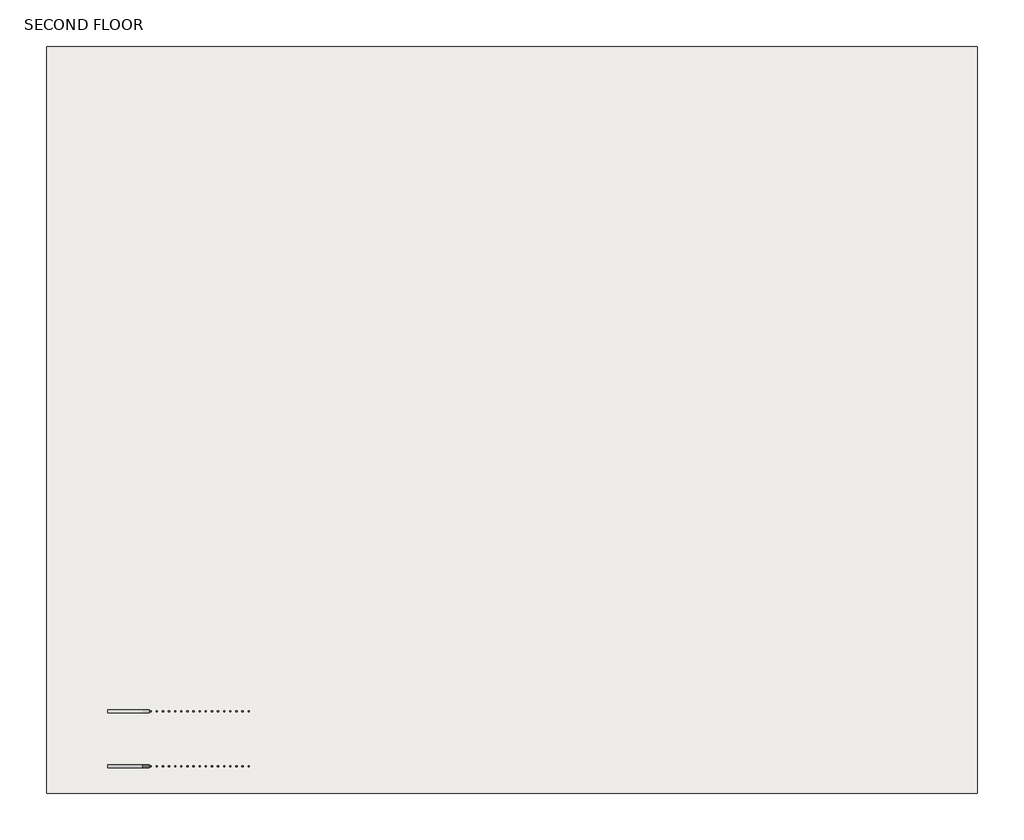
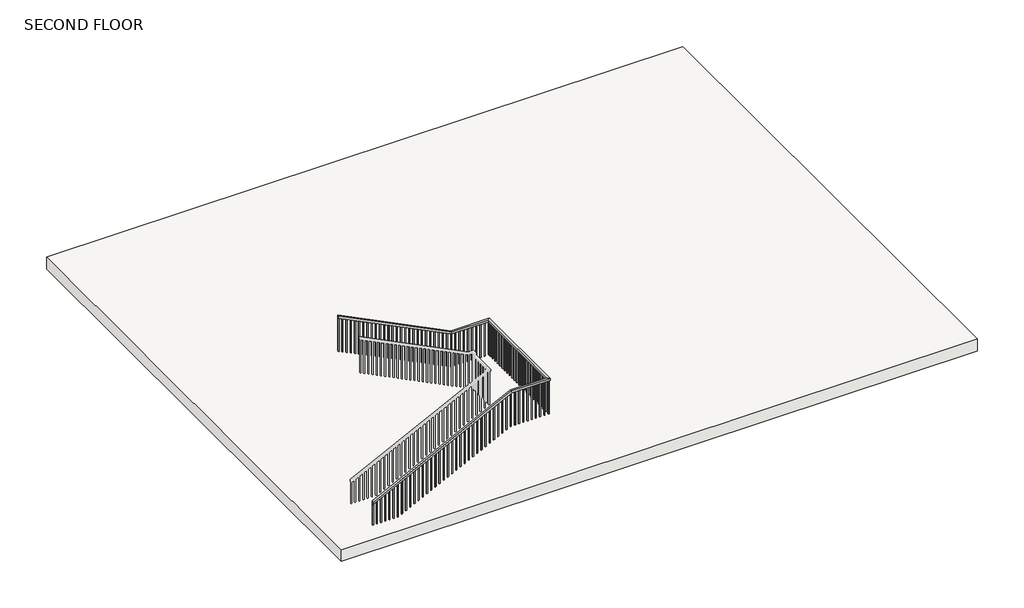
# One storey, part 1 of 2: 1 railing, 1 slab.
"""IFC4 building model written with IfcOpenShell, lengths in millimetres."""

from ifc_helpers import new_model, si_unit, frame, origin, place, context, project, spatial, polyline, outline, extrude, faceted_brep, element, save

model = new_model("IFC4")

# Units and contexts
model_context = context("Model", 3, world=origin())
ifc_project = project(units=[si_unit("LENGTHUNIT", "METRE", prefix="MILLI")], contexts=[model_context])

# Site, building, storey
site = spatial("IfcSite", under=ifc_project)
building = spatial("IfcBuilding", under=site)
storey = spatial("IfcBuildingStorey", under=building, Name="SECOND FLOOR", Elevation=6096.0)

# Railing
placement = place(None, origin())
element("IfcRailing", 1, ObjectType="Handrail - Rectangular", at=placement, inside=storey, context=model_context, shape_type="SolidModel", body=[
    faceted_brep([(-8362.2800418, -5370.1090076, 7010.4), (-8362.2800418, -5370.1090076, 6953.6038734), (-8362.2800418, -5420.9090076, 6953.6038734), (-8362.2800418, -5420.9090076, 7010.4), (-5009.4800418, -5370.1090076, 8686.8), (-4997.4877885, -5370.1090076, 8636.0), (-4997.4877885, -5420.9090076, 8636.0), (-5009.4800418, -5420.9090076, 8686.8), (-4120.4800418, -5370.1090076, 8686.8), (-4120.4800418, -5370.1090076, 8636.0), (-4069.6800418, -5420.9090076, 8636.0), (-4069.6800418, -5420.9090076, 8686.8), (-4120.4800418, -2917.1346494, 8686.8), (-4120.4800418, -2917.1346494, 8636.0), (-4069.6800418, -2866.3346494, 8636.0), (-4069.6800418, -2866.3346494, 8686.8), (-5009.4800418, -2917.1346494, 8686.8), (-5021.472295, -2917.1346494, 8636.0), (-5021.472295, -2866.3346494, 8636.0), (-5009.4800418, -2866.3346494, 8686.8), (-7752.6800418, -2917.1346494, 10058.4), (-7752.6800418, -2866.3346494, 10058.4), (-7752.6800418, -2866.3346494, 10001.6038734), (-7752.6800418, -2917.1346494, 10001.6038734)], [[[0, 1, 2, 3]], [[1, 0, 4, 5]], [[2, 1, 5, 6]], [[3, 2, 6, 7]], [[0, 3, 7, 4]], [[5, 4, 8, 9]], [[6, 5, 9, 10]], [[7, 6, 10, 11]], [[4, 7, 11, 8]], [[9, 8, 12, 13]], [[10, 9, 13, 14]], [[11, 10, 14, 15]], [[8, 11, 15, 12]], [[13, 12, 16, 17]], [[14, 13, 17, 18]], [[15, 14, 18, 19]], [[12, 15, 19, 16]], [[20, 21, 22, 23]], [[17, 16, 20, 23]], [[18, 17, 23, 22]], [[19, 18, 22, 21]], [[16, 19, 21, 20]]]),
    extrude(outline(polyline([(9955.5663734, -7660.6050418), (9097.9625, -7660.6050418), (9088.4375, -7641.5550418), (9946.0413734, -7641.5550418), (9955.5663734, -7660.6050418)])), frame((0.0, -2901.2596494, 0.0), z_axis=(0.0, 1.0, 0.0), x_axis=(0.0, 0.0, 1.0)), (0.0, 0.0, 1.0), 19.05),
    extrude(outline(polyline([(9904.7663734, -7559.0050418), (9047.1625, -7559.0050418), (9037.6375, -7539.9550418), (9895.2413734, -7539.9550418), (9904.7663734, -7559.0050418)])), frame((0.0, -2901.2596494, 0.0), z_axis=(0.0, 1.0, 0.0), x_axis=(0.0, 0.0, 1.0)), (0.0, 0.0, 1.0), 19.05),
    extrude(outline(polyline([(9853.9663734, -7457.4050418), (8996.3625, -7457.4050418), (8986.8375, -7438.3550418), (9844.4413734, -7438.3550418), (9853.9663734, -7457.4050418)])), frame((0.0, -2901.2596494, 0.0), z_axis=(0.0, 1.0, 0.0), x_axis=(0.0, 0.0, 1.0)), (0.0, 0.0, 1.0), 19.05),
    extrude(outline(polyline([(9803.1663734, -7355.8050418), (8945.5625, -7355.8050418), (8936.0375, -7336.7550418), (9793.6413734, -7336.7550418), (9803.1663734, -7355.8050418)])), frame((0.0, -2901.2596494, 0.0), z_axis=(0.0, 1.0, 0.0), x_axis=(0.0, 0.0, 1.0)), (0.0, 0.0, 1.0), 19.05),
    extrude(outline(polyline([(9752.3663734, -7254.2050418), (8894.7625, -7254.2050418), (8885.2375, -7235.1550418), (9742.8413734, -7235.1550418), (9752.3663734, -7254.2050418)])), frame((0.0, -2901.2596494, 0.0), z_axis=(0.0, 1.0, 0.0), x_axis=(0.0, 0.0, 1.0)), (0.0, 0.0, 1.0), 19.05),
    extrude(outline(polyline([(9701.5663734, -7152.6050418), (8843.9625, -7152.6050418), (8834.4375, -7133.5550418), (9692.0413734, -7133.5550418), (9701.5663734, -7152.6050418)])), frame((0.0, -2901.2596494, 0.0), z_axis=(0.0, 1.0, 0.0), x_axis=(0.0, 0.0, 1.0)), (0.0, 0.0, 1.0), 19.05),
    extrude(outline(polyline([(9650.7663734, -7051.0050418), (8793.1625, -7051.0050418), (8783.6375, -7031.9550418), (9641.2413734, -7031.9550418), (9650.7663734, -7051.0050418)])), frame((0.0, -2901.2596494, 0.0), z_axis=(0.0, 1.0, 0.0), x_axis=(0.0, 0.0, 1.0)), (0.0, 0.0, 1.0), 19.05),
    extrude(outline(polyline([(9599.9663734, -6949.4050418), (8742.3625, -6949.4050418), (8732.8375, -6930.3550418), (9590.4413734, -6930.3550418), (9599.9663734, -6949.4050418)])), frame((0.0, -2901.2596494, 0.0), z_axis=(0.0, 1.0, 0.0), x_axis=(0.0, 0.0, 1.0)), (0.0, 0.0, 1.0), 19.05),
    extrude(outline(polyline([(9549.1663734, -6847.8050418), (8691.5625, -6847.8050418), (8682.0375, -6828.7550418), (9539.6413734, -6828.7550418), (9549.1663734, -6847.8050418)])), frame((0.0, -2901.2596494, 0.0), z_axis=(0.0, 1.0, 0.0), x_axis=(0.0, 0.0, 1.0)), (0.0, 0.0, 1.0), 19.05),
    extrude(outline(polyline([(9498.3663734, -6746.2050418), (8640.7625, -6746.2050418), (8631.2375, -6727.1550418), (9488.8413734, -6727.1550418), (9498.3663734, -6746.2050418)])), frame((0.0, -2901.2596494, 0.0), z_axis=(0.0, 1.0, 0.0), x_axis=(0.0, 0.0, 1.0)), (0.0, 0.0, 1.0), 19.05),
    extrude(outline(polyline([(9447.5663734, -6644.6050418), (8589.9625, -6644.6050418), (8580.4375, -6625.5550418), (9438.0413734, -6625.5550418), (9447.5663734, -6644.6050418)])), frame((0.0, -2901.2596494, 0.0), z_axis=(0.0, 1.0, 0.0), x_axis=(0.0, 0.0, 1.0)), (0.0, 0.0, 1.0), 19.05),
    extrude(outline(polyline([(9396.7663734, -6543.0050418), (8539.1625, -6543.0050418), (8529.6375, -6523.9550418), (9387.2413734, -6523.9550418), (9396.7663734, -6543.0050418)])), frame((0.0, -2901.2596494, 0.0), z_axis=(0.0, 1.0, 0.0), x_axis=(0.0, 0.0, 1.0)), (0.0, 0.0, 1.0), 19.05),
    extrude(outline(polyline([(9345.9663734, -6441.4050418), (8488.3625, -6441.4050418), (8478.8375, -6422.3550418), (9336.4413734, -6422.3550418), (9345.9663734, -6441.4050418)])), frame((0.0, -2901.2596494, 0.0), z_axis=(0.0, 1.0, 0.0), x_axis=(0.0, 0.0, 1.0)), (0.0, 0.0, 1.0), 19.05),
    extrude(outline(polyline([(9295.1663734, -6339.8050418), (8437.5625, -6339.8050418), (8428.0375, -6320.7550418), (9285.6413734, -6320.7550418), (9295.1663734, -6339.8050418)])), frame((0.0, -2901.2596494, 0.0), z_axis=(0.0, 1.0, 0.0), x_axis=(0.0, 0.0, 1.0)), (0.0, 0.0, 1.0), 19.05),
    extrude(outline(polyline([(9244.3663734, -6238.2050418), (8386.7625, -6238.2050418), (8377.2375, -6219.1550418), (9234.8413734, -6219.1550418), (9244.3663734, -6238.2050418)])), frame((0.0, -2901.2596494, 0.0), z_axis=(0.0, 1.0, 0.0), x_axis=(0.0, 0.0, 1.0)), (0.0, 0.0, 1.0), 19.05),
    extrude(outline(polyline([(9193.5663734, -6136.6050418), (8335.9625, -6136.6050418), (8326.4375, -6117.5550418), (9184.0413734, -6117.5550418), (9193.5663734, -6136.6050418)])), frame((0.0, -2901.2596494, 0.0), z_axis=(0.0, 1.0, 0.0), x_axis=(0.0, 0.0, 1.0)), (0.0, 0.0, 1.0), 19.05),
    extrude(outline(polyline([(9142.7663734, -6035.0050418), (8285.1625, -6035.0050418), (8275.6375, -6015.9550418), (9133.2413734, -6015.9550418), (9142.7663734, -6035.0050418)])), frame((0.0, -2901.2596494, 0.0), z_axis=(0.0, 1.0, 0.0), x_axis=(0.0, 0.0, 1.0)), (0.0, 0.0, 1.0), 19.05),
    extrude(outline(polyline([(9091.9663734, -5933.4050418), (8234.3625, -5933.4050418), (8224.8375, -5914.3550418), (9082.4413734, -5914.3550418), (9091.9663734, -5933.4050418)])), frame((0.0, -2901.2596494, 0.0), z_axis=(0.0, 1.0, 0.0), x_axis=(0.0, 0.0, 1.0)), (0.0, 0.0, 1.0), 19.05),
    extrude(outline(polyline([(9041.1663734, -5831.8050418), (8183.5625, -5831.8050418), (8174.0375, -5812.7550418), (9031.6413734, -5812.7550418), (9041.1663734, -5831.8050418)])), frame((0.0, -2901.2596494, 0.0), z_axis=(0.0, 1.0, 0.0), x_axis=(0.0, 0.0, 1.0)), (0.0, 0.0, 1.0), 19.05),
    extrude(outline(polyline([(8990.3663734, -5730.2050418), (8132.7625, -5730.2050418), (8123.2375, -5711.1550418), (8980.8413734, -5711.1550418), (8990.3663734, -5730.2050418)])), frame((0.0, -2901.2596494, 0.0), z_axis=(0.0, 1.0, 0.0), x_axis=(0.0, 0.0, 1.0)), (0.0, 0.0, 1.0), 19.05),
    extrude(outline(polyline([(8939.5663734, -5628.6050418), (8081.9625, -5628.6050418), (8072.4375, -5609.5550418), (8930.0413734, -5609.5550418), (8939.5663734, -5628.6050418)])), frame((0.0, -2901.2596494, 0.0), z_axis=(0.0, 1.0, 0.0), x_axis=(0.0, 0.0, 1.0)), (0.0, 0.0, 1.0), 19.05),
    extrude(outline(polyline([(8888.7663734, -5527.0050418), (8031.1625, -5527.0050418), (8021.6375, -5507.9550418), (8879.2413734, -5507.9550418), (8888.7663734, -5527.0050418)])), frame((0.0, -2901.2596494, 0.0), z_axis=(0.0, 1.0, 0.0), x_axis=(0.0, 0.0, 1.0)), (0.0, 0.0, 1.0), 19.05),
    extrude(outline(polyline([(8837.9663734, -5425.4050418), (7980.3625, -5425.4050418), (7970.8375, -5406.3550418), (8828.4413734, -5406.3550418), (8837.9663734, -5425.4050418)])), frame((0.0, -2901.2596494, 0.0), z_axis=(0.0, 1.0, 0.0), x_axis=(0.0, 0.0, 1.0)), (0.0, 0.0, 1.0), 19.05),
    extrude(outline(polyline([(8787.1663734, -5323.8050418), (7929.5625, -5323.8050418), (7920.0375, -5304.7550418), (8777.6413734, -5304.7550418), (8787.1663734, -5323.8050418)])), frame((0.0, -2901.2596494, 0.0), z_axis=(0.0, 1.0, 0.0), x_axis=(0.0, 0.0, 1.0)), (0.0, 0.0, 1.0), 19.05),
    extrude(outline(polyline([(8736.3663734, -5222.2050418), (7878.7625, -5222.2050418), (7869.2375, -5203.1550418), (8726.8413734, -5203.1550418), (8736.3663734, -5222.2050418)])), frame((0.0, -2901.2596494, 0.0), z_axis=(0.0, 1.0, 0.0), x_axis=(0.0, 0.0, 1.0)), (0.0, 0.0, 1.0), 19.05),
    extrude(outline(polyline([(8685.5663734, -5120.6050418), (7827.9625, -5120.6050418), (7818.4375, -5101.5550418), (8676.0413734, -5101.5550418), (8685.5663734, -5120.6050418)])), frame((0.0, -2901.2596494, 0.0), z_axis=(0.0, 1.0, 0.0), x_axis=(0.0, 0.0, 1.0)), (0.0, 0.0, 1.0), 19.05),
    extrude(outline(polyline([(-4898.3550418, -2901.2596494), (-4917.4050418, -2901.2596494), (-4917.4050418, -2882.2096494), (-4898.3550418, -2882.2096494), (-4898.3550418, -2901.2596494)])), frame((0.0, 0.0, 7772.4), z_axis=(0.0, 0.0, 1.0), x_axis=(1.0, 0.0, 0.0)), (0.0, 0.0, 1.0), 863.6),
    extrude(outline(polyline([(-4796.7550418, -2901.2596494), (-4815.8050418, -2901.2596494), (-4815.8050418, -2882.2096494), (-4796.7550418, -2882.2096494), (-4796.7550418, -2901.2596494)])), frame((0.0, 0.0, 7772.4), z_axis=(0.0, 0.0, 1.0), x_axis=(1.0, 0.0, 0.0)), (0.0, 0.0, 1.0), 863.6),
    extrude(outline(polyline([(-4695.1550418, -2901.2596494), (-4714.2050418, -2901.2596494), (-4714.2050418, -2882.2096494), (-4695.1550418, -2882.2096494), (-4695.1550418, -2901.2596494)])), frame((0.0, 0.0, 7772.4), z_axis=(0.0, 0.0, 1.0), x_axis=(1.0, 0.0, 0.0)), (0.0, 0.0, 1.0), 863.6),
    extrude(outline(polyline([(-4593.5550418, -2901.2596494), (-4612.6050418, -2901.2596494), (-4612.6050418, -2882.2096494), (-4593.5550418, -2882.2096494), (-4593.5550418, -2901.2596494)])), frame((0.0, 0.0, 7772.4), z_axis=(0.0, 0.0, 1.0), x_axis=(1.0, 0.0, 0.0)), (0.0, 0.0, 1.0), 863.6),
    extrude(outline(polyline([(-4491.9550418, -2901.2596494), (-4511.0050418, -2901.2596494), (-4511.0050418, -2882.2096494), (-4491.9550418, -2882.2096494), (-4491.9550418, -2901.2596494)])), frame((0.0, 0.0, 7772.4), z_axis=(0.0, 0.0, 1.0), x_axis=(1.0, 0.0, 0.0)), (0.0, 0.0, 1.0), 863.6),
    extrude(outline(polyline([(-4390.3550418, -2901.2596494), (-4409.4050418, -2901.2596494), (-4409.4050418, -2882.2096494), (-4390.3550418, -2882.2096494), (-4390.3550418, -2901.2596494)])), frame((0.0, 0.0, 7772.4), z_axis=(0.0, 0.0, 1.0), x_axis=(1.0, 0.0, 0.0)), (0.0, 0.0, 1.0), 863.6),
    extrude(outline(polyline([(-4288.7550418, -2901.2596494), (-4307.8050418, -2901.2596494), (-4307.8050418, -2882.2096494), (-4288.7550418, -2882.2096494), (-4288.7550418, -2901.2596494)])), frame((0.0, 0.0, 7772.4), z_axis=(0.0, 0.0, 1.0), x_axis=(1.0, 0.0, 0.0)), (0.0, 0.0, 1.0), 863.6),
    extrude(outline(polyline([(-4187.1550418, -2901.2596494), (-4206.2050418, -2901.2596494), (-4206.2050418, -2882.2096494), (-4187.1550418, -2882.2096494), (-4187.1550418, -2901.2596494)])), frame((0.0, 0.0, 7772.4), z_axis=(0.0, 0.0, 1.0), x_axis=(1.0, 0.0, 0.0)), (0.0, 0.0, 1.0), 863.6),
    extrude(outline(polyline([(-4104.6050418, -2966.6340076), (-4104.6050418, -2947.5840076), (-4085.5550418, -2947.5840076), (-4085.5550418, -2966.6340076), (-4104.6050418, -2966.6340076)])), frame((0.0, 0.0, 7772.4), z_axis=(0.0, 0.0, 1.0), x_axis=(1.0, 0.0, 0.0)), (0.0, 0.0, 1.0), 863.6),
    extrude(outline(polyline([(-4104.6050418, -3068.2340076), (-4104.6050418, -3049.1840076), (-4085.5550418, -3049.1840076), (-4085.5550418, -3068.2340076), (-4104.6050418, -3068.2340076)])), frame((0.0, 0.0, 7772.4), z_axis=(0.0, 0.0, 1.0), x_axis=(1.0, 0.0, 0.0)), (0.0, 0.0, 1.0), 863.6),
    extrude(outline(polyline([(-4104.6050418, -3169.8340076), (-4104.6050418, -3150.7840076), (-4085.5550418, -3150.7840076), (-4085.5550418, -3169.8340076), (-4104.6050418, -3169.8340076)])), frame((0.0, 0.0, 7772.4), z_axis=(0.0, 0.0, 1.0), x_axis=(1.0, 0.0, 0.0)), (0.0, 0.0, 1.0), 863.6),
    extrude(outline(polyline([(-4104.6050418, -3271.4340076), (-4104.6050418, -3252.3840076), (-4085.5550418, -3252.3840076), (-4085.5550418, -3271.4340076), (-4104.6050418, -3271.4340076)])), frame((0.0, 0.0, 7772.4), z_axis=(0.0, 0.0, 1.0), x_axis=(1.0, 0.0, 0.0)), (0.0, 0.0, 1.0), 863.6),
    extrude(outline(polyline([(-4104.6050418, -3373.0340076), (-4104.6050418, -3353.9840076), (-4085.5550418, -3353.9840076), (-4085.5550418, -3373.0340076), (-4104.6050418, -3373.0340076)])), frame((0.0, 0.0, 7772.4), z_axis=(0.0, 0.0, 1.0), x_axis=(1.0, 0.0, 0.0)), (0.0, 0.0, 1.0), 863.6),
    extrude(outline(polyline([(-4104.6050418, -3474.6340076), (-4104.6050418, -3455.5840076), (-4085.5550418, -3455.5840076), (-4085.5550418, -3474.6340076), (-4104.6050418, -3474.6340076)])), frame((0.0, 0.0, 7772.4), z_axis=(0.0, 0.0, 1.0), x_axis=(1.0, 0.0, 0.0)), (0.0, 0.0, 1.0), 863.6),
    extrude(outline(polyline([(-4104.6050418, -3576.2340076), (-4104.6050418, -3557.1840076), (-4085.5550418, -3557.1840076), (-4085.5550418, -3576.2340076), (-4104.6050418, -3576.2340076)])), frame((0.0, 0.0, 7772.4), z_axis=(0.0, 0.0, 1.0), x_axis=(1.0, 0.0, 0.0)), (0.0, 0.0, 1.0), 863.6),
    extrude(outline(polyline([(-4104.6050418, -3677.8340076), (-4104.6050418, -3658.7840076), (-4085.5550418, -3658.7840076), (-4085.5550418, -3677.8340076), (-4104.6050418, -3677.8340076)])), frame((0.0, 0.0, 7772.4), z_axis=(0.0, 0.0, 1.0), x_axis=(1.0, 0.0, 0.0)), (0.0, 0.0, 1.0), 863.6),
    extrude(outline(polyline([(-4104.6050418, -3779.4340076), (-4104.6050418, -3760.3840076), (-4085.5550418, -3760.3840076), (-4085.5550418, -3779.4340076), (-4104.6050418, -3779.4340076)])), frame((0.0, 0.0, 7772.4), z_axis=(0.0, 0.0, 1.0), x_axis=(1.0, 0.0, 0.0)), (0.0, 0.0, 1.0), 863.6),
    extrude(outline(polyline([(-4104.6050418, -3881.0340076), (-4104.6050418, -3861.9840076), (-4085.5550418, -3861.9840076), (-4085.5550418, -3881.0340076), (-4104.6050418, -3881.0340076)])), frame((0.0, 0.0, 7772.4), z_axis=(0.0, 0.0, 1.0), x_axis=(1.0, 0.0, 0.0)), (0.0, 0.0, 1.0), 863.6),
    extrude(outline(polyline([(-4104.6050418, -3982.6340076), (-4104.6050418, -3963.5840076), (-4085.5550418, -3963.5840076), (-4085.5550418, -3982.6340076), (-4104.6050418, -3982.6340076)])), frame((0.0, 0.0, 7772.4), z_axis=(0.0, 0.0, 1.0), x_axis=(1.0, 0.0, 0.0)), (0.0, 0.0, 1.0), 863.6),
    extrude(outline(polyline([(-4104.6050418, -4084.2340076), (-4104.6050418, -4065.1840076), (-4085.5550418, -4065.1840076), (-4085.5550418, -4084.2340076), (-4104.6050418, -4084.2340076)])), frame((0.0, 0.0, 7772.4), z_axis=(0.0, 0.0, 1.0), x_axis=(1.0, 0.0, 0.0)), (0.0, 0.0, 1.0), 863.6),
    extrude(outline(polyline([(-4104.6050418, -4185.8340076), (-4104.6050418, -4166.7840076), (-4085.5550418, -4166.7840076), (-4085.5550418, -4185.8340076), (-4104.6050418, -4185.8340076)])), frame((0.0, 0.0, 7772.4), z_axis=(0.0, 0.0, 1.0), x_axis=(1.0, 0.0, 0.0)), (0.0, 0.0, 1.0), 863.6),
    extrude(outline(polyline([(-4104.6050418, -4287.4340076), (-4104.6050418, -4268.3840076), (-4085.5550418, -4268.3840076), (-4085.5550418, -4287.4340076), (-4104.6050418, -4287.4340076)])), frame((0.0, 0.0, 7772.4), z_axis=(0.0, 0.0, 1.0), x_axis=(1.0, 0.0, 0.0)), (0.0, 0.0, 1.0), 863.6),
    extrude(outline(polyline([(-4104.6050418, -4389.0340076), (-4104.6050418, -4369.9840076), (-4085.5550418, -4369.9840076), (-4085.5550418, -4389.0340076), (-4104.6050418, -4389.0340076)])), frame((0.0, 0.0, 7772.4), z_axis=(0.0, 0.0, 1.0), x_axis=(1.0, 0.0, 0.0)), (0.0, 0.0, 1.0), 863.6),
    extrude(outline(polyline([(-4104.6050418, -4490.6340076), (-4104.6050418, -4471.5840076), (-4085.5550418, -4471.5840076), (-4085.5550418, -4490.6340076), (-4104.6050418, -4490.6340076)])), frame((0.0, 0.0, 7772.4), z_axis=(0.0, 0.0, 1.0), x_axis=(1.0, 0.0, 0.0)), (0.0, 0.0, 1.0), 863.6),
    extrude(outline(polyline([(-4104.6050418, -4592.2340076), (-4104.6050418, -4573.1840076), (-4085.5550418, -4573.1840076), (-4085.5550418, -4592.2340076), (-4104.6050418, -4592.2340076)])), frame((0.0, 0.0, 7772.4), z_axis=(0.0, 0.0, 1.0), x_axis=(1.0, 0.0, 0.0)), (0.0, 0.0, 1.0), 863.6),
    extrude(outline(polyline([(-4104.6050418, -4693.8340076), (-4104.6050418, -4674.7840076), (-4085.5550418, -4674.7840076), (-4085.5550418, -4693.8340076), (-4104.6050418, -4693.8340076)])), frame((0.0, 0.0, 7772.4), z_axis=(0.0, 0.0, 1.0), x_axis=(1.0, 0.0, 0.0)), (0.0, 0.0, 1.0), 863.6),
    extrude(outline(polyline([(-4104.6050418, -4795.4340076), (-4104.6050418, -4776.3840076), (-4085.5550418, -4776.3840076), (-4085.5550418, -4795.4340076), (-4104.6050418, -4795.4340076)])), frame((0.0, 0.0, 7772.4), z_axis=(0.0, 0.0, 1.0), x_axis=(1.0, 0.0, 0.0)), (0.0, 0.0, 1.0), 863.6),
    extrude(outline(polyline([(-4104.6050418, -4897.0340076), (-4104.6050418, -4877.9840076), (-4085.5550418, -4877.9840076), (-4085.5550418, -4897.0340076), (-4104.6050418, -4897.0340076)])), frame((0.0, 0.0, 7772.4), z_axis=(0.0, 0.0, 1.0), x_axis=(1.0, 0.0, 0.0)), (0.0, 0.0, 1.0), 863.6),
    extrude(outline(polyline([(-4104.6050418, -4998.6340076), (-4104.6050418, -4979.5840076), (-4085.5550418, -4979.5840076), (-4085.5550418, -4998.6340076), (-4104.6050418, -4998.6340076)])), frame((0.0, 0.0, 7772.4), z_axis=(0.0, 0.0, 1.0), x_axis=(1.0, 0.0, 0.0)), (0.0, 0.0, 1.0), 863.6),
    extrude(outline(polyline([(-4104.6050418, -5100.2340076), (-4104.6050418, -5081.1840076), (-4085.5550418, -5081.1840076), (-4085.5550418, -5100.2340076), (-4104.6050418, -5100.2340076)])), frame((0.0, 0.0, 7772.4), z_axis=(0.0, 0.0, 1.0), x_axis=(1.0, 0.0, 0.0)), (0.0, 0.0, 1.0), 863.6),
    extrude(outline(polyline([(-4104.6050418, -5201.8340076), (-4104.6050418, -5182.7840076), (-4085.5550418, -5182.7840076), (-4085.5550418, -5201.8340076), (-4104.6050418, -5201.8340076)])), frame((0.0, 0.0, 7772.4), z_axis=(0.0, 0.0, 1.0), x_axis=(1.0, 0.0, 0.0)), (0.0, 0.0, 1.0), 863.6),
    extrude(outline(polyline([(-4104.6050418, -5303.4340076), (-4104.6050418, -5284.3840076), (-4085.5550418, -5284.3840076), (-4085.5550418, -5303.4340076), (-4104.6050418, -5303.4340076)])), frame((0.0, 0.0, 7772.4), z_axis=(0.0, 0.0, 1.0), x_axis=(1.0, 0.0, 0.0)), (0.0, 0.0, 1.0), 863.6),
    extrude(outline(polyline([(-4206.2050418, -5385.9840076), (-4187.1550418, -5385.9840076), (-4187.1550418, -5405.0340076), (-4206.2050418, -5405.0340076), (-4206.2050418, -5385.9840076)])), frame((0.0, 0.0, 7772.4), z_axis=(0.0, 0.0, 1.0), x_axis=(1.0, 0.0, 0.0)), (0.0, 0.0, 1.0), 863.6),
    extrude(outline(polyline([(-4307.8050418, -5385.9840076), (-4288.7550418, -5385.9840076), (-4288.7550418, -5405.0340076), (-4307.8050418, -5405.0340076), (-4307.8050418, -5385.9840076)])), frame((0.0, 0.0, 7772.4), z_axis=(0.0, 0.0, 1.0), x_axis=(1.0, 0.0, 0.0)), (0.0, 0.0, 1.0), 863.6),
    extrude(outline(polyline([(-4409.4050418, -5385.9840076), (-4390.3550418, -5385.9840076), (-4390.3550418, -5405.0340076), (-4409.4050418, -5405.0340076), (-4409.4050418, -5385.9840076)])), frame((0.0, 0.0, 7772.4), z_axis=(0.0, 0.0, 1.0), x_axis=(1.0, 0.0, 0.0)), (0.0, 0.0, 1.0), 863.6),
    extrude(outline(polyline([(-4511.0050418, -5385.9840076), (-4491.9550418, -5385.9840076), (-4491.9550418, -5405.0340076), (-4511.0050418, -5405.0340076), (-4511.0050418, -5385.9840076)])), frame((0.0, 0.0, 7772.4), z_axis=(0.0, 0.0, 1.0), x_axis=(1.0, 0.0, 0.0)), (0.0, 0.0, 1.0), 863.6),
    extrude(outline(polyline([(-4612.6050418, -5385.9840076), (-4593.5550418, -5385.9840076), (-4593.5550418, -5405.0340076), (-4612.6050418, -5405.0340076), (-4612.6050418, -5385.9840076)])), frame((0.0, 0.0, 7772.4), z_axis=(0.0, 0.0, 1.0), x_axis=(1.0, 0.0, 0.0)), (0.0, 0.0, 1.0), 863.6),
    extrude(outline(polyline([(-4714.2050418, -5385.9840076), (-4695.1550418, -5385.9840076), (-4695.1550418, -5405.0340076), (-4714.2050418, -5405.0340076), (-4714.2050418, -5385.9840076)])), frame((0.0, 0.0, 7772.4), z_axis=(0.0, 0.0, 1.0), x_axis=(1.0, 0.0, 0.0)), (0.0, 0.0, 1.0), 863.6),
    extrude(outline(polyline([(-4815.8050418, -5385.9840076), (-4796.7550418, -5385.9840076), (-4796.7550418, -5405.0340076), (-4815.8050418, -5405.0340076), (-4815.8050418, -5385.9840076)])), frame((0.0, 0.0, 7772.4), z_axis=(0.0, 0.0, 1.0), x_axis=(1.0, 0.0, 0.0)), (0.0, 0.0, 1.0), 863.6),
    extrude(outline(polyline([(-4917.4050418, -5385.9840076), (-4898.3550418, -5385.9840076), (-4898.3550418, -5405.0340076), (-4917.4050418, -5405.0340076), (-4917.4050418, -5385.9840076)])), frame((0.0, 0.0, 7772.4), z_axis=(0.0, 0.0, 1.0), x_axis=(1.0, 0.0, 0.0)), (0.0, 0.0, 1.0), 863.6),
    extrude(outline(polyline([(8574.4413734, -5120.6050418), (7716.8375, -5120.6050418), (7726.3625, -5101.5550418), (8583.9663734, -5101.5550418), (8574.4413734, -5120.6050418)])), frame((0.0, -5405.0340076, 0.0), z_axis=(0.0, 1.0, 0.0), x_axis=(0.0, 0.0, 1.0)), (0.0, 0.0, 1.0), 19.05),
    extrude(outline(polyline([(8523.6413734, -5222.2050418), (7666.0375, -5222.2050418), (7675.5625, -5203.1550418), (8533.1663734, -5203.1550418), (8523.6413734, -5222.2050418)])), frame((0.0, -5405.0340076, 0.0), z_axis=(0.0, 1.0, 0.0), x_axis=(0.0, 0.0, 1.0)), (0.0, 0.0, 1.0), 19.05),
    extrude(outline(polyline([(8472.8413734, -5323.8050418), (7615.2375, -5323.8050418), (7624.7625, -5304.7550418), (8482.3663734, -5304.7550418), (8472.8413734, -5323.8050418)])), frame((0.0, -5405.0340076, 0.0), z_axis=(0.0, 1.0, 0.0), x_axis=(0.0, 0.0, 1.0)), (0.0, 0.0, 1.0), 19.05),
    extrude(outline(polyline([(8422.0413734, -5425.4050418), (7564.4375, -5425.4050418), (7573.9625, -5406.3550418), (8431.5663734, -5406.3550418), (8422.0413734, -5425.4050418)])), frame((0.0, -5405.0340076, 0.0), z_axis=(0.0, 1.0, 0.0), x_axis=(0.0, 0.0, 1.0)), (0.0, 0.0, 1.0), 19.05),
    extrude(outline(polyline([(8371.2413734, -5527.0050418), (7513.6375, -5527.0050418), (7523.1625, -5507.9550418), (8380.7663734, -5507.9550418), (8371.2413734, -5527.0050418)])), frame((0.0, -5405.0340076, 0.0), z_axis=(0.0, 1.0, 0.0), x_axis=(0.0, 0.0, 1.0)), (0.0, 0.0, 1.0), 19.05),
    extrude(outline(polyline([(8320.4413734, -5628.6050418), (7462.8375, -5628.6050418), (7472.3625, -5609.5550418), (8329.9663734, -5609.5550418), (8320.4413734, -5628.6050418)])), frame((0.0, -5405.0340076, 0.0), z_axis=(0.0, 1.0, 0.0), x_axis=(0.0, 0.0, 1.0)), (0.0, 0.0, 1.0), 19.05),
    extrude(outline(polyline([(8269.6413734, -5730.2050418), (7412.0375, -5730.2050418), (7421.5625, -5711.1550418), (8279.1663734, -5711.1550418), (8269.6413734, -5730.2050418)])), frame((0.0, -5405.0340076, 0.0), z_axis=(0.0, 1.0, 0.0), x_axis=(0.0, 0.0, 1.0)), (0.0, 0.0, 1.0), 19.05),
    extrude(outline(polyline([(8218.8413734, -5831.8050418), (7361.2375, -5831.8050418), (7370.7625, -5812.7550418), (8228.3663734, -5812.7550418), (8218.8413734, -5831.8050418)])), frame((0.0, -5405.0340076, 0.0), z_axis=(0.0, 1.0, 0.0), x_axis=(0.0, 0.0, 1.0)), (0.0, 0.0, 1.0), 19.05),
    extrude(outline(polyline([(8168.0413734, -5933.4050418), (7310.4375, -5933.4050418), (7319.9625, -5914.3550418), (8177.5663734, -5914.3550418), (8168.0413734, -5933.4050418)])), frame((0.0, -5405.0340076, 0.0), z_axis=(0.0, 1.0, 0.0), x_axis=(0.0, 0.0, 1.0)), (0.0, 0.0, 1.0), 19.05),
    extrude(outline(polyline([(8117.2413734, -6035.0050418), (7259.6375, -6035.0050418), (7269.1625, -6015.9550418), (8126.7663734, -6015.9550418), (8117.2413734, -6035.0050418)])), frame((0.0, -5405.0340076, 0.0), z_axis=(0.0, 1.0, 0.0), x_axis=(0.0, 0.0, 1.0)), (0.0, 0.0, 1.0), 19.05),
    extrude(outline(polyline([(8066.4413734, -6136.6050418), (7208.8375, -6136.6050418), (7218.3625, -6117.5550418), (8075.9663734, -6117.5550418), (8066.4413734, -6136.6050418)])), frame((0.0, -5405.0340076, 0.0), z_axis=(0.0, 1.0, 0.0), x_axis=(0.0, 0.0, 1.0)), (0.0, 0.0, 1.0), 19.05),
    extrude(outline(polyline([(8015.6413734, -6238.2050418), (7158.0375, -6238.2050418), (7167.5625, -6219.1550418), (8025.1663734, -6219.1550418), (8015.6413734, -6238.2050418)])), frame((0.0, -5405.0340076, 0.0), z_axis=(0.0, 1.0, 0.0), x_axis=(0.0, 0.0, 1.0)), (0.0, 0.0, 1.0), 19.05),
    extrude(outline(polyline([(7964.8413734, -6339.8050418), (7107.2375, -6339.8050418), (7116.7625, -6320.7550418), (7974.3663734, -6320.7550418), (7964.8413734, -6339.8050418)])), frame((0.0, -5405.0340076, 0.0), z_axis=(0.0, 1.0, 0.0), x_axis=(0.0, 0.0, 1.0)), (0.0, 0.0, 1.0), 19.05),
    extrude(outline(polyline([(7914.0413734, -6441.4050418), (7056.4375, -6441.4050418), (7065.9625, -6422.3550418), (7923.5663734, -6422.3550418), (7914.0413734, -6441.4050418)])), frame((0.0, -5405.0340076, 0.0), z_axis=(0.0, 1.0, 0.0), x_axis=(0.0, 0.0, 1.0)), (0.0, 0.0, 1.0), 19.05),
    extrude(outline(polyline([(7863.2413734, -6543.0050418), (7005.6375, -6543.0050418), (7015.1625, -6523.9550418), (7872.7663734, -6523.9550418), (7863.2413734, -6543.0050418)])), frame((0.0, -5405.0340076, 0.0), z_axis=(0.0, 1.0, 0.0), x_axis=(0.0, 0.0, 1.0)), (0.0, 0.0, 1.0), 19.05),
    extrude(outline(polyline([(7812.4413734, -6644.6050418), (6954.8375, -6644.6050418), (6964.3625, -6625.5550418), (7821.9663734, -6625.5550418), (7812.4413734, -6644.6050418)])), frame((0.0, -5405.0340076, 0.0), z_axis=(0.0, 1.0, 0.0), x_axis=(0.0, 0.0, 1.0)), (0.0, 0.0, 1.0), 19.05),
    extrude(outline(polyline([(7761.6413734, -6746.2050418), (6904.0375, -6746.2050418), (6913.5625, -6727.1550418), (7771.1663734, -6727.1550418), (7761.6413734, -6746.2050418)])), frame((0.0, -5405.0340076, 0.0), z_axis=(0.0, 1.0, 0.0), x_axis=(0.0, 0.0, 1.0)), (0.0, 0.0, 1.0), 19.05),
    extrude(outline(polyline([(7710.8413734, -6847.8050418), (6853.2375, -6847.8050418), (6862.7625, -6828.7550418), (7720.3663734, -6828.7550418), (7710.8413734, -6847.8050418)])), frame((0.0, -5405.0340076, 0.0), z_axis=(0.0, 1.0, 0.0), x_axis=(0.0, 0.0, 1.0)), (0.0, 0.0, 1.0), 19.05),
    extrude(outline(polyline([(7660.0413734, -6949.4050418), (6802.4375, -6949.4050418), (6811.9625, -6930.3550418), (7669.5663734, -6930.3550418), (7660.0413734, -6949.4050418)])), frame((0.0, -5405.0340076, 0.0), z_axis=(0.0, 1.0, 0.0), x_axis=(0.0, 0.0, 1.0)), (0.0, 0.0, 1.0), 19.05),
    extrude(outline(polyline([(7609.2413734, -7051.0050418), (6751.6375, -7051.0050418), (6761.1625, -7031.9550418), (7618.7663734, -7031.9550418), (7609.2413734, -7051.0050418)])), frame((0.0, -5405.0340076, 0.0), z_axis=(0.0, 1.0, 0.0), x_axis=(0.0, 0.0, 1.0)), (0.0, 0.0, 1.0), 19.05),
    extrude(outline(polyline([(7558.4413734, -7152.6050418), (6700.8375, -7152.6050418), (6710.3625, -7133.5550418), (7567.9663734, -7133.5550418), (7558.4413734, -7152.6050418)])), frame((0.0, -5405.0340076, 0.0), z_axis=(0.0, 1.0, 0.0), x_axis=(0.0, 0.0, 1.0)), (0.0, 0.0, 1.0), 19.05),
    extrude(outline(polyline([(7507.6413734, -7254.2050418), (6650.0375, -7254.2050418), (6659.5625, -7235.1550418), (7517.1663734, -7235.1550418), (7507.6413734, -7254.2050418)])), frame((0.0, -5405.0340076, 0.0), z_axis=(0.0, 1.0, 0.0), x_axis=(0.0, 0.0, 1.0)), (0.0, 0.0, 1.0), 19.05),
    extrude(outline(polyline([(7456.8413734, -7355.8050418), (6599.2375, -7355.8050418), (6608.7625, -7336.7550418), (7466.3663734, -7336.7550418), (7456.8413734, -7355.8050418)])), frame((0.0, -5405.0340076, 0.0), z_axis=(0.0, 1.0, 0.0), x_axis=(0.0, 0.0, 1.0)), (0.0, 0.0, 1.0), 19.05),
    extrude(outline(polyline([(7406.0413734, -7457.4050418), (6548.4375, -7457.4050418), (6557.9625, -7438.3550418), (7415.5663734, -7438.3550418), (7406.0413734, -7457.4050418)])), frame((0.0, -5405.0340076, 0.0), z_axis=(0.0, 1.0, 0.0), x_axis=(0.0, 0.0, 1.0)), (0.0, 0.0, 1.0), 19.05),
    extrude(outline(polyline([(7355.2413734, -7559.0050418), (6497.6375, -7559.0050418), (6507.1625, -7539.9550418), (7364.7663734, -7539.9550418), (7355.2413734, -7559.0050418)])), frame((0.0, -5405.0340076, 0.0), z_axis=(0.0, 1.0, 0.0), x_axis=(0.0, 0.0, 1.0)), (0.0, 0.0, 1.0), 19.05),
    extrude(outline(polyline([(7304.4413734, -7660.6050418), (6446.8375, -7660.6050418), (6456.3625, -7641.5550418), (7313.9663734, -7641.5550418), (7304.4413734, -7660.6050418)])), frame((0.0, -5405.0340076, 0.0), z_axis=(0.0, 1.0, 0.0), x_axis=(0.0, 0.0, 1.0)), (0.0, 0.0, 1.0), 19.05),
    extrude(outline(polyline([(7253.6413734, -7762.2050418), (6396.0375, -7762.2050418), (6405.5625, -7743.1550418), (7263.1663734, -7743.1550418), (7253.6413734, -7762.2050418)])), frame((0.0, -5405.0340076, 0.0), z_axis=(0.0, 1.0, 0.0), x_axis=(0.0, 0.0, 1.0)), (0.0, 0.0, 1.0), 19.05),
    extrude(outline(polyline([(7202.8413734, -7863.8050418), (6345.2375, -7863.8050418), (6354.7625, -7844.7550418), (7212.3663734, -7844.7550418), (7202.8413734, -7863.8050418)])), frame((0.0, -5405.0340076, 0.0), z_axis=(0.0, 1.0, 0.0), x_axis=(0.0, 0.0, 1.0)), (0.0, 0.0, 1.0), 19.05),
    extrude(outline(polyline([(7152.0413734, -7965.4050418), (6294.4375, -7965.4050418), (6303.9625, -7946.3550418), (7161.5663734, -7946.3550418), (7152.0413734, -7965.4050418)])), frame((0.0, -5405.0340076, 0.0), z_axis=(0.0, 1.0, 0.0), x_axis=(0.0, 0.0, 1.0)), (0.0, 0.0, 1.0), 19.05),
    extrude(outline(polyline([(7101.2413734, -8067.0050418), (6243.6375, -8067.0050418), (6253.1625, -8047.9550418), (7110.7663734, -8047.9550418), (7101.2413734, -8067.0050418)])), frame((0.0, -5405.0340076, 0.0), z_axis=(0.0, 1.0, 0.0), x_axis=(0.0, 0.0, 1.0)), (0.0, 0.0, 1.0), 19.05),
    extrude(outline(polyline([(7050.4413734, -8168.6050418), (6192.8375, -8168.6050418), (6202.3625, -8149.5550418), (7059.9663734, -8149.5550418), (7050.4413734, -8168.6050418)])), frame((0.0, -5405.0340076, 0.0), z_axis=(0.0, 1.0, 0.0), x_axis=(0.0, 0.0, 1.0)), (0.0, 0.0, 1.0), 19.05),
    extrude(outline(polyline([(6999.6413734, -8270.2050418), (6142.0375, -8270.2050418), (6151.5625, -8251.1550418), (7009.1663734, -8251.1550418), (6999.6413734, -8270.2050418)])), frame((0.0, -5405.0340076, 0.0), z_axis=(0.0, 1.0, 0.0), x_axis=(0.0, 0.0, 1.0)), (0.0, 0.0, 1.0), 19.05),
    extrude(outline(polyline([(-4999.9550418, -2901.2596494), (-5019.0050418, -2901.2596494), (-5019.0050418, -2882.2096494), (-4999.9550418, -2882.2096494), (-4999.9550418, -2901.2596494)])), frame((0.0, 0.0, 7772.4), z_axis=(0.0, 0.0, 1.0), x_axis=(1.0, 0.0, 0.0)), (0.0, 0.0, 1.0), 863.6),
    extrude(outline(polyline([(-4104.6050418, -2901.2596494), (-4104.6050418, -2882.2096494), (-4085.5550418, -2882.2096494), (-4085.5550418, -2901.2596494), (-4104.6050418, -2901.2596494)])), frame((0.0, 0.0, 7772.4), z_axis=(0.0, 0.0, 1.0), x_axis=(1.0, 0.0, 0.0)), (0.0, 0.0, 1.0), 863.6),
    extrude(outline(polyline([(-4104.6050418, -5385.9840076), (-4085.5550418, -5385.9840076), (-4085.5550418, -5405.0340076), (-4104.6050418, -5405.0340076), (-4104.6050418, -5385.9840076)])), frame((0.0, 0.0, 7772.4), z_axis=(0.0, 0.0, 1.0), x_axis=(1.0, 0.0, 0.0)), (0.0, 0.0, 1.0), 863.6),
    extrude(outline(polyline([(8625.2413734, -5019.0050418), (7767.6375, -5019.0050418), (7777.1625, -4999.9550418), (8634.7663734, -4999.9550418), (8625.2413734, -5019.0050418)])), frame((0.0, -5405.0340076, 0.0), z_axis=(0.0, 1.0, 0.0), x_axis=(0.0, 0.0, 1.0)), (0.0, 0.0, 1.0), 19.05),
    extrude(outline(polyline([(10001.6038734, -7752.6800418), (9144.0, -7752.6800418), (9134.475, -7733.6300418), (9992.0788734, -7733.6300418), (10001.6038734, -7752.6800418)])), frame((0.0, -2901.2596494, 0.0), z_axis=(0.0, 1.0, 0.0), x_axis=(0.0, 0.0, 1.0)), (0.0, 0.0, 1.0), 19.05),
    extrude(outline(polyline([(6953.6038734, -8362.2800418), (6096.0, -8362.2800418), (6105.525, -8343.2300418), (6963.1288734, -8343.2300418), (6953.6038734, -8362.2800418)])), frame((0.0, -5405.0340076, 0.0), z_axis=(0.0, 1.0, 0.0), x_axis=(0.0, 0.0, 1.0)), (0.0, 0.0, 1.0), 19.05),
])

# Slab
element("IfcSlab", 2, ObjectType="Generic - 12\"", at=placement, inside=storey, context=model_context, shape_type="SweptSolid", body=[
    extrude(outline(polyline([(6064.2982466, 6554.3761968), (6064.2982466, -5840.8238032), (-9378.9017534, -5840.8238032), (-9378.9017534, 6554.3761968), (6064.2982466, 6554.3761968)])), frame((0.0, 0.0, 6096.0), z_axis=(0.0, 0.0, 1.0), x_axis=(1.0, 0.0, 0.0)), (0.0, 0.0, 1.0), 304.8),
])

save(model, "model.ifc")

# Revit data of these elements
# Type "Handrail - Rectangular"
#   Assembly Code = "C2010400"
#   built-in parameter 1008612 = 0.0416667 (stored number, unit not read)
#   built-in parameter 1008611 = 0.0416667 (stored number, unit not read)
#   built-in parameter 1008609 = 0.333333 (stored number, unit not read)
#   built-in parameter 1008604 = 0.166667 (stored number, unit not read)
#   built-in parameter 1008603 = 0.166667 (stored number, unit not read)
#   Railing Height = 3' - 0"
#   built-in parameter 1008630 = 2
#   built-in parameter 1008610 = 2
#   built-in parameter 1008618 = Baluster - Square : 3/4"
# Type "Generic - 12\""
#   Assembly Code = "B1010"
#   Function = 0
#   Layers, outside or top first: 1' - 0" no material (function 1)
# Element 1 (IfcRailing, "Handrail - Rectangular")
#   Phase Created = New Construction
# Element 2 (IfcSlab, "Generic - 12\"")
#   Height Offset From Level = 1' - 0"
#   Phase Created = New Construction
#   Materials on its faces: "Default Floor"
# Materials
#   "Default Floor": colour RGB 128 128 128, transparency 0, Cost = 0
